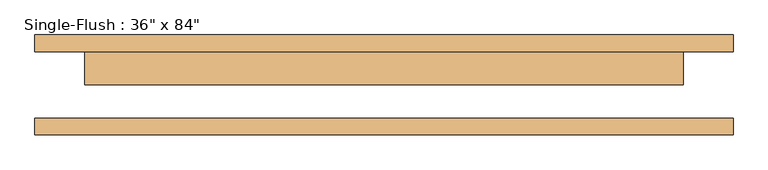
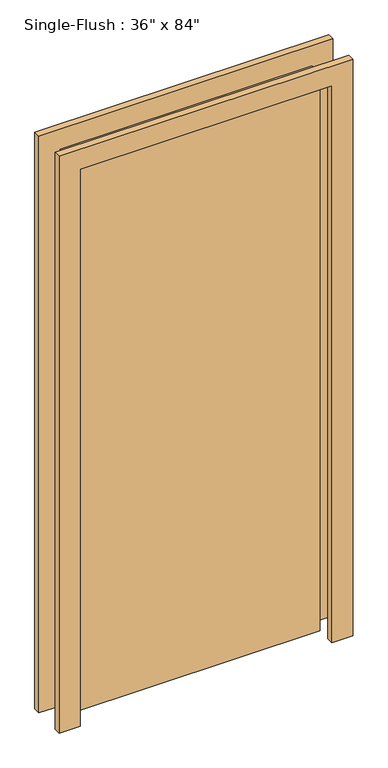
"""IFC4 building model written with IfcOpenShell, lengths in millimetres: door geometry."""

from ifc_helpers import new_model, si_unit, frame, origin, origin_with_axes, place, context, project, spatial, polyline, outline, extrude, source, transform, mapped, element, save


def door_048588e9(model_context):
    return source(origin(), model_context, "Body", "SweptSolid", [
        extrude(outline(polyline([(2209.8, -533.4), (0.0, -533.4), (0.0, -457.2), (2133.6, -457.2), (2133.6, 457.2), (0.0, 457.2), (0.0, 533.4), (2209.8, 533.4), (2209.8, -533.4)])), frame((0.0, 50.8, 0.0), z_axis=(0.0, 1.0, 0.0), x_axis=(0.0, 0.0, 1.0)), (0.0, 0.0, 1.0), 25.4),
        extrude(outline(polyline([(2209.8, 533.4), (2209.8, -533.4), (0.0, -533.4), (0.0, -457.2), (2133.6, -457.2), (2133.6, 457.2), (0.0, 457.2), (0.0, 533.4), (2209.8, 533.4)])), frame((0.0, -76.2, 0.0), z_axis=(0.0, 1.0, 0.0), x_axis=(0.0, 0.0, 1.0)), (0.0, 0.0, 1.0), 25.4),
        extrude(outline(polyline([(457.2, 0.0), (-457.2, 0.0), (-457.2, 50.8), (457.2, 50.8), (457.2, 0.0)])), origin_with_axes(), (0.0, 0.0, 1.0), 2133.6),
    ])


if __name__ == "__main__":
    model = new_model("IFC4")
    model_context = context("Model", 3, world=origin())
    ifc_project = project(units=[si_unit("LENGTHUNIT", "METRE", prefix="MILLI")], contexts=[model_context])
    site = spatial("IfcSite", under=ifc_project)
    building = spatial("IfcBuilding", under=site)
    placement = place(None, origin())
    door_shape = door_048588e9(model_context)
    element("IfcDoor", 1, ObjectType="Single-Flush : 36\" x 84\"", at=placement, inside=building, context=model_context, shape_type="MappedRepresentation", body=[
        mapped(door_shape, transform((0.0, 0.0, 0.0), x_axis=(1.0, 0.0, 0.0), y_axis=(0.0, 1.0, 0.0), z_axis=(0.0, 0.0, 1.0))),
    ])
    save(model, "model.ifc")

# Revit data of these elements
# Type "Single-Flush : 36\" x 84\""
#   Type Mark = "5"
#   Construction Type Id = "MDOOR"
#   Assembly Code = "C1020"
#   Analytic Construction = "Metal"
#   Thickness = 0' - 2"
#   Heat Transfer Coefficient (U) = 0.651978 BTU/(h·ft²·°F)
#   Height = 7' - 0"
#   Trim Projection Ext = 0' - 1"
#   Trim Projection Int = 0' - 1"
#   Trim Width = 0' - 3"
#   Width = 3' - 0"
#   Define Thermal Properties by = 1
#   Define Thermal Properties by = 1
#   Door Material = Door - Panel
#   Frame Material = Door - Frame
#   Visual Light Transmittance = 0
#   Solar Heat Gain Coefficient = 0
#   Function = (empty or 0)
#   Wall Closure = (empty or 0)
# Element 1 (IfcDoor, "Single-Flush : 36\" x 84\"")
#   Materials on its faces: "Door - Frame", "Door - Panel"
# Materials
#   "Door - Panel": class "Wood", colour RGB 210 159 95, transparency 0, Cost = 0
#   "Door - Frame": colour RGB 118 70 51, transparency 0, Cost = 0
